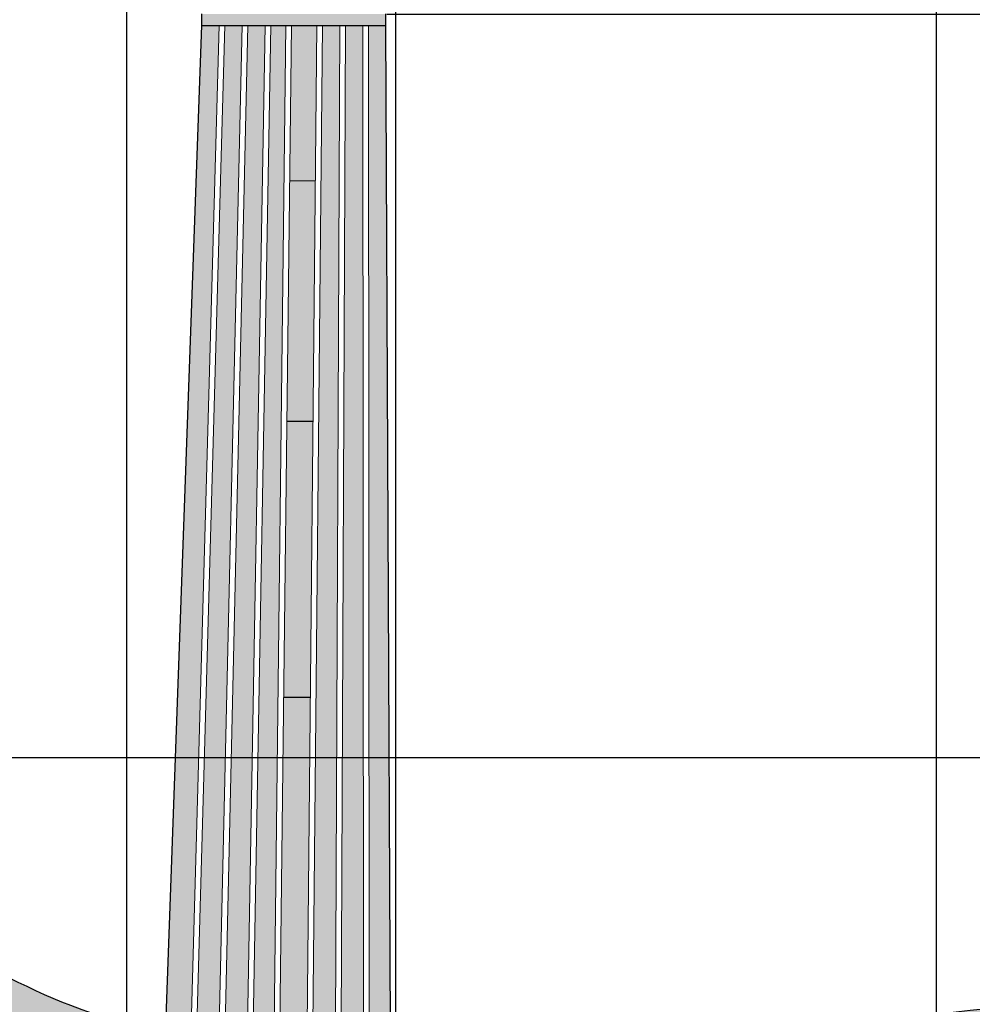
# Model space of a CAD drawing. Units: millimetres. Extents: x 11032 to 26788, y 3406 to 24505.
# Tile 76 of 78: x 16895 to 21051, y 17443 to 21738. Entities that reach past the tile are written whole.
import ezdxf

# ---------------------------------------------------------------- set-up
doc = ezdxf.new("R2010")
doc.units = ezdxf.units.MM
doc.header["$MEASUREMENT"] = 0
for name, color, linetype, lineweight in [('A-ANNO-DIMS', 2, 'Continuous', 18), ('A-ELEV-NECK', 7, 'Continuous', 25), ('A-ELEV-STRG', 7, 'Continuous', 13), ('A-ROOF', 7, 'Continuous', 30)]:
    doc.layers.add(name, color=color, linetype=linetype, lineweight=lineweight)
for name, color, linetype, lineweight, true_color in [('A-ELEV-NECK-PATT', 159, 'Continuous', 13, 0x22346e), ('A-ELEV-TUNE-PATT', 251, 'Continuous', 13, 0x636466), ('A-ROOF-PATT', 9, 'Continuous', 13, 0xc7c8ca)]:
    doc.layers.add(name, color=color, linetype=linetype, lineweight=lineweight, true_color=true_color)
doc.styles.get("Standard").update_dxf_attribs({"font": 'arial.ttf'})
doc.dimstyles.get("Standard").update_dxf_attribs({"dimtxt": 150, "dimasz": 100, "dimexe": 10, "dimexo": 5, "dimgap": 5, "dimtad": 0, "dimtih": 1, "dimtoh": 1, "dimdec": 0, "dimzin": 0, "dimdsep": 46, "dimtxsty": 'Standard', "dimcen": 0.09, "dimadec": 0, "dimazin": 0, "dimtfac": 1, "dimtdec": 0, "dimtofl": 0, "dimtmove": 0, "dimatfit": 3, "dimfxl": 1, "dimtolj": 1, "dimtzin": 0, "dimarcsym": 0})

# ---------------------------------------------------------------- blocks, each defined once
blk = doc.blocks.new('*D28')
at = {"layer": 'A-ANNO-DIMS', "color": 0, "lineweight": -2, "transparency": 16777216}
for p, q in [((17252.8, 22072.2), (17252.8, 22172.2)), ((17252.8, 22172.2), (17352.8, 22172.2)), ((17289.8, 22072.2), (17242.8, 22072.2)), ((17252.8, 21892.4), (17252.8, 21972.2)), ((17289.8, 21792.4), (17242.8, 21792.4))]:
    blk.add_line(p, q, dxfattribs=at)
at = {"layer": 'A-ANNO-DIMS', "color": 0, "transparency": 16777216}
for points in [[(17236.2, 21972.2), (17269.5, 21972.2), (17252.8, 22072.2)], [(17236.2, 21892.4), (17269.5, 21892.4), (17252.8, 21792.4)]]:
    blk.add_solid(points, dxfattribs=at)
at = {"layer": 'Defpoints', "color": 0, "transparency": 16777216}
for p in [(17252.8, 22072.2), (17294.8, 22072.2), (17294.8, 21792.4)]:
    blk.add_point(p, dxfattribs=at)
at = {"layer": 'A-ANNO-DIMS', "color": 0, "transparency": 16777216, "insert": (18452.5, 22172.2), "char_height": 150, "attachment_point": 5}
blk.add_mtext('\\A1;TUNING KEY 280 TYP.', dxfattribs=at)
blk = doc.blocks.new('*D36')
at = {"layer": 'A-ANNO-DIMS', "color": 0, "lineweight": -2, "transparency": 16777216}
for p, q in [((12301.3, 17115.9), (12301.3, 24416.9)), ((12401.3, 24406.9), (18569.2, 24406.9)), ((25297.4, 24406.9), (19129.5, 24406.9)), ((25397.4, 4466.4), (25397.4, 24416.9))]:
    blk.add_line(p, q, dxfattribs=at)
at = {"layer": 'A-ANNO-DIMS', "color": 0, "transparency": 16777216}
for points in [[(12401.3, 24423.5), (12401.3, 24390.2), (12301.3, 24406.9)], [(25297.4, 24423.5), (25297.4, 24390.2), (25397.4, 24406.9)]]:
    blk.add_solid(points, dxfattribs=at)
at = {"layer": 'Defpoints', "color": 0, "transparency": 16777216}
for p in [(25397.4, 24406.9), (12301.3, 17110.9), (25397.4, 4461.4)]:
    blk.add_point(p, dxfattribs=at)
at = {"layer": 'A-ANNO-DIMS', "color": 0, "transparency": 16777216, "insert": (18849.3, 24406.9), "char_height": 150, "attachment_point": 5}
blk.add_mtext('\\A1;13096', dxfattribs=at)
blk = doc.blocks.new('*D37')
at = {"layer": 'A-ANNO-DIMS', "color": 0, "lineweight": -2, "transparency": 16777216}
for p, q in [((18087.7, 23450.4), (11334.8, 23450.4)), ((11344.8, 23350.4), (11344.8, 14037.5)), ((11344.8, 4561.4), (11344.8, 13874.3)), ((12927.7, 4461.4), (11334.8, 4461.4))]:
    blk.add_line(p, q, dxfattribs=at)
at = {"layer": 'A-ANNO-DIMS', "color": 0, "transparency": 16777216}
for points in [[(11328.1, 23350.4), (11361.4, 23350.4), (11344.8, 23450.4)], [(11328.1, 4561.4), (11361.4, 4561.4), (11344.8, 4461.4)]]:
    blk.add_solid(points, dxfattribs=at)
at = {"layer": 'Defpoints', "color": 0, "transparency": 16777216}
for p in [(11344.8, 23450.4), (18092.7, 23450.4), (12932.7, 4461.4)]:
    blk.add_point(p, dxfattribs=at)
at = {"layer": 'A-ANNO-DIMS', "color": 0, "transparency": 16777216, "insert": (11344.8, 13955.9), "char_height": 150, "attachment_point": 5}
blk.add_mtext('\\A1;18989', dxfattribs=at)
blk = doc.blocks.new('*D45')
at = {"layer": 'A-ANNO-DIMS', "color": 0, "lineweight": -2, "transparency": 16777216}
for p, q in [((13792.4, 18518.9), (26363.9, 18518.9)), ((26353.9, 18418.9), (26353.9, 17450.3)), ((26353.9, 16318.4), (26353.9, 17287)), ((22902.4, 16218.4), (26363.9, 16218.4))]:
    blk.add_line(p, q, dxfattribs=at)
at = {"layer": 'A-ANNO-DIMS', "color": 0, "transparency": 16777216}
for points in [[(26337.2, 18418.9), (26370.6, 18418.9), (26353.9, 18518.9)], [(26337.2, 16318.4), (26370.6, 16318.4), (26353.9, 16218.4)]]:
    blk.add_solid(points, dxfattribs=at)
at = {"layer": 'Defpoints', "color": 0, "transparency": 16777216}
for p in [(13787.4, 18518.9), (26353.9, 18518.9), (22897.4, 16218.4)]:
    blk.add_point(p, dxfattribs=at)
at = {"layer": 'A-ANNO-DIMS', "color": 0, "transparency": 16777216, "insert": (26353.9, 17368.7), "char_height": 150, "attachment_point": 5}
blk.add_mtext('\\A1;2300.5', dxfattribs=at)
blk = doc.blocks.new('*D46')
at = {"layer": 'A-ANNO-DIMS', "color": 0, "lineweight": -2, "transparency": 16777216}
for p, q in [((18497.2, 21762.9), (26363.9, 21762.9)), ((26353.9, 21662.9), (26353.9, 20222.6)), ((26353.9, 18618.9), (26353.9, 20059.3)), ((13792.4, 18518.9), (26363.9, 18518.9))]:
    blk.add_line(p, q, dxfattribs=at)
at = {"layer": 'A-ANNO-DIMS', "color": 0, "transparency": 16777216}
for points in [[(26337.2, 21662.9), (26370.6, 21662.9), (26353.9, 21762.9)], [(26337.2, 18618.9), (26370.6, 18618.9), (26353.9, 18518.9)]]:
    blk.add_solid(points, dxfattribs=at)
at = {"layer": 'Defpoints', "color": 0, "transparency": 16777216}
for p in [(18492.2, 21762.9), (26353.9, 21762.9), (13787.4, 18518.9)]:
    blk.add_point(p, dxfattribs=at)
at = {"layer": 'A-ANNO-DIMS', "color": 0, "transparency": 16777216, "insert": (26353.9, 20140.9), "char_height": 150, "attachment_point": 5}
blk.add_mtext('\\A1;3244', dxfattribs=at)
blk = doc.blocks.new('*D57')
at = {"layer": 'A-ANNO-DIMS', "color": 0, "lineweight": -2, "transparency": 16777216}
for p, q in [((14994.7, 7266.4), (14994.7, 24416.9)), ((15094.7, 24406.9), (17716, 24406.9)), ((20794.7, 24406.9), (18173.4, 24406.9)), ((20894.7, 7266.4), (20894.7, 24416.9))]:
    blk.add_line(p, q, dxfattribs=at)
at = {"layer": 'A-ANNO-DIMS', "color": 0, "transparency": 16777216}
for points in [[(15094.7, 24423.5), (15094.7, 24390.2), (14994.7, 24406.9)], [(20794.7, 24423.5), (20794.7, 24390.2), (20894.7, 24406.9)]]:
    blk.add_solid(points, dxfattribs=at)
at = {"layer": 'Defpoints', "color": 0, "transparency": 16777216}
for p in [(20894.7, 24406.9), (14994.7, 7261.4), (20894.7, 7261.4)]:
    blk.add_point(p, dxfattribs=at)
at = {"layer": 'A-ANNO-DIMS', "color": 0, "transparency": 16777216, "insert": (17944.7, 24406.9), "char_height": 150, "attachment_point": 5}
blk.add_mtext('\\A1;5900', dxfattribs=at)
blk = doc.blocks.new('*D65')
at = {"layer": 'A-ANNO-DIMS', "color": 0, "lineweight": -2, "transparency": 16777216}
for p, q in [((17362, 12566.3), (17362, 24416.9)), ((17462, 24406.9), (17639.4, 24406.9)), ((18435.4, 24406.9), (18258, 24406.9)), ((18535.4, 12566.5), (18535.4, 24416.9))]:
    blk.add_line(p, q, dxfattribs=at)
at = {"layer": 'A-ANNO-DIMS', "color": 0, "transparency": 16777216}
for points in [[(17462, 24423.5), (17462, 24390.2), (17362, 24406.9)], [(18435.4, 24423.5), (18435.4, 24390.2), (18535.4, 24406.9)]]:
    blk.add_solid(points, dxfattribs=at)
at = {"layer": 'Defpoints', "color": 0, "transparency": 16777216}
for p in [(18535.4, 24406.9), (17362, 12561.3), (18535.4, 12561.5)]:
    blk.add_point(p, dxfattribs=at)
at = {"layer": 'A-ANNO-DIMS', "color": 0, "transparency": 16777216, "insert": (17948.7, 24406.9), "char_height": 150, "attachment_point": 5}
blk.add_mtext('\\A1;1173.3', dxfattribs=at)

msp = doc.modelspace()

# ---------------------------------------------------------------- hatches: boundary and pattern name
at = {"layer": 'A-ELEV-NECK-PATT'}
h = msp.add_hatch(color=256, dxfattribs=at)
h.set_gradient(color1=(82, 15, 16), color2=(153, 76, 0), name='INVHEMISPHERICAL')
edge = h.paths.add_edge_path()
edge.add_line((17765.577, 21712.945), (17690.161, 21712.945))
edge.add_line((17690.161, 21712.945), (17532.827, 17324.837))
edge.add_spline(control_points=[(17532.827, 17324.837), (17568.929, 17318.668), (17605.243, 17313.31), (17641.798, 17308.706)], knot_values=[8560.66857913, 8560.66857913, 8560.66857913, 8560.66857913, 8678.18536837, 8678.18536837, 8678.18536837, 8678.18536837], degree=3, periodic=0)
edge.add_line((17641.798, 17308.706), (17765.577, 21712.945))
edge = h.paths.add_edge_path()
edge.add_spline(control_points=[(17666.718, 17305.687), (17699.249, 17301.903), (17731.975, 17298.702), (17764.917, 17296.043)], knot_values=[8704.84912349, 8704.84912349, 8704.84912349, 8704.84912349, 8809.1081873, 8809.1081873, 8809.1081873, 8809.1081873], degree=3, periodic=0)
edge.add_line((17764.917, 17296.043), (17865.857, 21712.945))
edge.add_line((17865.857, 21712.945), (17790.586, 21712.945))
edge.add_line((17790.586, 21712.945), (17666.718, 17305.687))
edge = h.paths.add_edge_path()
edge.add_line((17966.114, 21712.945), (17890.863, 21712.945))
edge.add_line((17890.863, 21712.945), (17789.878, 17294.135))
edge.add_spline(control_points=[(17789.878, 17294.135), (17822.446, 17291.782), (17855.23, 17289.947), (17888.249, 17288.59)], knot_values=[8835.39626479, 8835.39626479, 8835.39626479, 8835.39626479, 8938.12522047, 8938.12522047, 8938.12522047, 8938.12522047], degree=3, periodic=0)
edge.add_line((17888.249, 17288.59), (17966.114, 21712.945))
h = msp.add_hatch(color=256, dxfattribs=at)
h.set_gradient(color1=(82, 15, 16), color2=(153, 76, 0), name='INVHEMISPHERICAL')
edge = h.paths.add_edge_path()
edge.add_line((18055.913, 21712.945), (17991.118, 21712.945))
edge.add_line((17991.118, 21712.945), (17913.235, 17287.655))
edge.add_spline(control_points=[(17913.235, 17287.655), (17923.7, 17287.302), (17934.19, 17286.996), (17944.704, 17286.735)], knot_values=[8963.99017486, 8963.99017486, 8963.99017486, 8963.99017486, 8996.4318779, 8996.4318779, 8996.4318779, 8996.4318779], degree=3, periodic=0)
edge.add_spline(control_points=[(17944.704, 17286.735), (17964.82, 17285.722), (17984.935, 17284.709), (18005.051, 17283.703)], knot_values=[0, 0, 0, 0, 60.41749209, 60.41749209, 60.41749209, 60.41749209], degree=3, periodic=0)
edge.add_line((18005.051, 17283.703), (18055.913, 21712.945))
edge = h.paths.add_edge_path()
edge.add_line((18492.19, 21712.945), (18416.998, 21712.945))
edge.add_line((18416.998, 21712.945), (18420.504, 17266.134))
edge.add_spline(control_points=[(18420.504, 17266.134), (18451.394, 17265.216), (18482.287, 17264.397), (18513.182, 17263.662)], knot_values=[476.26006783, 476.26006783, 476.26006783, 476.26006783, 568.98430855, 568.98430855, 568.98430855, 568.98430855], degree=3, periodic=0)
edge.add_line((18513.182, 17263.662), (18492.19, 21712.945))
edge = h.paths.add_edge_path()
edge.add_spline(control_points=[(18296.914, 17270.367), (18316.656, 17269.603), (18349.518, 17268.396), (18382.383, 17267.313), (18395.503, 17266.9)], knot_values=[352.58081587, 352.58081587, 352.58081587, 352.58081587, 411.85892504, 451.24395945, 451.24395945, 451.24395945, 451.24395945], degree=3, periodic=0)
edge.add_line((18395.503, 17266.9), (18391.999, 21712.945))
edge.add_line((18391.999, 21712.945), (18316.752, 21712.945))
edge.add_line((18316.752, 21712.945), (18296.914, 17270.367))
edge = h.paths.add_edge_path()
edge.add_line((18291.755, 21712.945), (18216.518, 21712.945))
edge.add_line((18216.518, 21712.945), (18173.381, 17275.594))
edge.add_spline(control_points=[(18173.381, 17275.594), (18206.225, 17274.101), (18239.071, 17272.678), (18271.92, 17271.355)], knot_values=[228.93242669, 228.93242669, 228.93242669, 228.93242669, 327.56540209, 327.56540209, 327.56540209, 327.56540209], degree=3, periodic=0)
edge.add_line((18271.92, 17271.355), (18291.755, 21712.945))
h = msp.add_hatch(color=256, dxfattribs=at)
h.set_gradient(color1=(82, 15, 16), color2=(153, 76, 0), name='INVCURVED')
h.paths.add_polyline_path([(18047.271, 18783.21), (18163.029, 18782.085), (18174.733, 19985.929), (18061.095, 19987.033)])
h.paths.add_polyline_path([(18184.929, 21034.754), (18073.138, 21035.841), (18061.095, 19987.033), (18174.733, 19985.929)])
h.paths.add_polyline_path([(18073.138, 21035.841), (18184.929, 21034.754), (18191.522, 21712.945), (18080.914, 21712.945)])
h = msp.add_hatch(color=256, dxfattribs=at)
h.set_gradient(color1=(82, 15, 16), color2=(153, 76, 0), name='INVCURVED')
edge = h.paths.add_edge_path()
edge.add_spline(control_points=[(18030.038, 17282.457), (18069.489, 17280.497), (18108.941, 17278.575), (18148.395, 17276.742)], knot_values=[85.43243603, 85.43243603, 85.43243603, 85.43243603, 203.92020001, 203.92020001, 203.92020001, 203.92020001], degree=3, periodic=0)
edge.add_line((18148.395, 17276.742), (18163.029, 18782.085))
edge.add_line((18163.029, 18782.085), (18047.271, 18783.21))
edge.add_line((18047.271, 18783.21), (18030.038, 17282.457))
at = {"layer": 'A-ELEV-TUNE-PATT'}
msp.add_hatch(color=256, dxfattribs=at).paths.add_polyline_path([(18492.19, 21762.945), (17690.161, 21762.945), (17690.161, 21712.945), (18055.913, 21712.945), (18055.916, 21713.232), (18492.19, 21712.945)])
at = {"layer": 'A-ROOF-PATT'}
h = msp.add_hatch(color=256, dxfattribs=at)
edge = h.paths.add_edge_path()
edge.add_spline(control_points=[(17532.827, 17324.837), (17391.335, 17349.016), (16840.872, 17494.912), (16080.055, 18069.544), (14738.803, 18299.641), (13382.429, 18838.336), (12580.532, 17870.207), (12430.422, 17563.822)], knot_values=[2977.60279446, 2977.60279446, 2977.60279446, 2977.60279446, 3438.18406011, 4811.64630219, 5622.86754827, 7588.02881883, 8560.66857913, 8560.66857913, 8560.66857913, 8560.66857913], degree=3, periodic=0)
edge.add_spline(control_points=[(12430.422, 17563.822), (12437.904, 17573.36), (12445.386, 17582.899), (12452.869, 17592.437), (12452.869, 17592.438), (12452.869, 17592.438), (12452.869, 17592.438)], knot_values=[1408.56413798, 1408.56413798, 1408.56413798, 1408.56413798, 1444.85989, 1444.85989, 1444.85989, 1444.86011829, 1444.86011829, 1444.86011829, 1444.86011829], degree=3, periodic=0)
edge.add_spline(control_points=[(12452.869, 17592.438), (12555.432, 17723.185), (12736.557, 17929.686), (13044.86, 18114.643), (13219.943, 18189.644), (13299.92, 18220.646)], knot_values=[339.31824597, 339.31824597, 339.31824597, 339.31824597, 836.83499673, 1151.25129334, 1408.56413798, 1408.56413798, 1408.56413798, 1408.56413798], degree=3, periodic=0)
edge.add_spline(control_points=[(13299.92, 18220.646), (13299.998, 18220.689), (13300.077, 18220.732), (13319.738, 18231.488), (13339.24, 18241.402), (13388.645, 18264.703), (13418.466, 18277.069), (13478.019, 18298.648), (13507.751, 18307.861), (13544.561, 18317.488), (13551.584, 18319.245), (13558.612, 18320.924)], knot_values=[3783.89509717, 3783.89509717, 3783.89509717, 3783.89509717, 3784.1737101, 3784.1737101, 3853.4666747, 3853.4666747, 3960.24019172, 3960.24019172, 4067.01370874, 4067.01370874, 4092.17446487, 4092.17446487, 4092.17446487, 4092.17446487], degree=3, periodic=0)
edge.add_spline(control_points=[(13558.612, 18320.924), (13581.407, 18326.373), (13604.25, 18331.007), (13657.184, 18339.957), (13687.338, 18343.732), (13748.098, 18348.892), (13778.704, 18350.276), (13840.46, 18350.833), (13871.609, 18350.005), (13934.496, 18346.313), (13966.232, 18343.449), (14030.297, 18335.871), (14062.625, 18331.158), (14127.853, 18320.088), (14160.753, 18313.73), (14241.357, 18296.556), (14289.343, 18284.997), (14386.31, 18259.688), (14435.291, 18245.941), (14534.161, 18217.034), (14584.049, 18201.875), (14684.682, 18170.964), (14735.427, 18155.212), (14837.763, 18123.971), (14889.354, 18108.482), (14954.971, 18089.677), (14968.586, 18085.823), (14992.391, 18079.184), (15002.566, 18076.376), (15021.739, 18071.153), (15030.731, 18068.729), (15047.707, 18064.21), (15055.694, 18062.106), (15079.815, 18055.825), (15095.905, 18051.728), (15143.966, 18039.717), (15175.729, 18032.084), (15254.84, 18013.501), (15301.798, 18002.866), (15394.186, 17981.845), (15439.615, 17971.459), (15528.833, 17950.135), (15572.62, 17939.197), (15658.477, 17916.021), (15700.546, 17903.785), (15753.633, 17886.734), (15765.446, 17882.835), (15786.574, 17875.653), (15795.915, 17872.404), (15810.108, 17867.349), (15814.99, 17865.588), (15824.736, 17862.029), (15829.611, 17860.226), (15844.241, 17854.75), (15854.002, 17851.008), (15883.312, 17839.521), (15902.885, 17831.512), (15966.355, 17804.548), (16010.39, 17784.302), (16098.838, 17741.267), (16143.25, 17718.478), (16232.497, 17671.098), (16277.332, 17646.507), (16367.515, 17596.295), (16412.862, 17570.676), (16504.202, 17519.209), (16550.194, 17493.362), (16643.009, 17442.263), (16689.831, 17417.011), (16756.517, 17382.472), (16775.937, 17372.58), (16795.455, 17362.84)], knot_values=[4092.17446487, 4092.17446487, 4092.17446487, 4092.17446487, 4173.78722577, 4173.78722577, 4280.56074279, 4280.56074279, 4387.33425981, 4387.33425981, 4494.10777683, 4494.10777683, 4600.88129386, 4600.88129386, 4707.65481088, 4707.65481088, 4814.4283279, 4814.4283279, 4967.12624049, 4967.12624049, 5119.82415308, 5119.82415308, 5272.52206566, 5272.52206566, 5425.21997825, 5425.21997825, 5577.91789084, 5577.91789084, 5617.78533194, 5617.78533194, 5647.46484794, 5647.46484794, 5673.61102495, 5673.61102495, 5696.74760695, 5696.74760695, 5743.68189033, 5743.68189033, 5837.55045709, 5837.55045709, 5979.72610459, 5979.72610459, 6121.90175208, 6121.90175208, 6264.07739957, 6264.07739957, 6406.25304706, 6406.25304706, 6447.25858494, 6447.25858494, 6480.04208821, 6480.04208821, 6497.30770621, 6497.30770621, 6514.5733242, 6514.5733242, 6549.10456019, 6549.10456019, 6618.16703217, 6618.16703217, 6772.66101707, 6772.66101707, 6927.15500198, 6927.15500198, 7081.64898689, 7081.64898689, 7236.1429718, 7236.1429718, 7390.6369567, 7390.6369567, 7545.13094161, 7545.13094161, 7608.19928683, 7608.19928683, 7608.19928683, 7608.19928683], degree=3, periodic=0)
edge.add_spline(control_points=[(16795.455, 17362.84), (16814.335, 17349.456), (16832.897, 17336.263), (16873.225, 17307.197), (16894.778, 17291.386), (16936.221, 17259.941), (16956.11, 17244.308), (16993.863, 17213.094), (17011.726, 17197.514), (17041.993, 17169.265), (17054.791, 17156.601), (17078.762, 17131.225), (17089.933, 17118.516), (17110.618, 17092.991), (17120.131, 17080.178), (17130.17, 17065.264), (17131.487, 17063.277), (17133.77, 17059.776), (17134.746, 17058.261), (17136.69, 17055.205), (17137.657, 17053.668), (17140.539, 17049.025), (17142.438, 17045.89), (17148.068, 17036.367), (17151.732, 17029.859), (17163.03, 17008.788), (17170.335, 16993.646), (17184.087, 16961.978), (17190.534, 16945.453), (17202.562, 16911.165), (17208.142, 16893.402), (17218.448, 16856.821), (17223.173, 16838.003), (17231.801, 16799.51), (17235.705, 16779.837), (17241.533, 16746.739), (17243.676, 16733.5), (17247.718, 16706.37), (17249.608, 16692.472), (17252.066, 16672.69), (17252.761, 16666.875), (17254.1, 16655.226), (17254.744, 16649.4), (17256.596, 16631.917), (17257.727, 16620.254), (17260.823, 16585.238), (17262.489, 16561.858), (17266.551, 16488.654), (17267.658, 16438.661), (17267.349, 16375.228), (17267.193, 16362.07), (17266.95, 16348.891)], knot_values=[15.11304723, 15.11304723, 15.11304723, 15.11304723, 82.69951457, 82.69951457, 165.39902914, 165.39902914, 248.09854371, 248.09854371, 330.79805828, 330.79805828, 397.94194582, 397.94194582, 465.08583335, 465.08583335, 532.22972088, 532.22972088, 542.53374101, 542.53374101, 550.35681582, 550.35681582, 558.17989062, 558.17989062, 573.82604024, 573.82604024, 605.11833946, 605.11833946, 672.76406143, 672.76406143, 740.4097834, 740.4097834, 808.05550537, 808.05550537, 875.70122735, 875.70122735, 943.34694932, 943.34694932, 987.66134917, 987.66134917, 1033.41216123, 1033.41216123, 1052.38508762, 1052.38508762, 1071.35801402, 1071.35801402, 1109.30386682, 1109.30386682, 1185.19557241, 1185.19557241, 1346.44190265, 1346.44190265, 1388.55866312, 1388.55866312, 1388.55866312, 1388.55866312], degree=3, periodic=0)
edge.add_spline(control_points=[(17266.95, 16348.891), (17266.95, 16348.891), (17266.95, 16348.891), (17266.95, 16348.891), (17253.182, 15602.417), (17239.414, 14855.943), (17225.646, 14109.469)], knot_values=[1388.55866312, 1388.55866312, 1388.55866312, 1388.55866312, 1388.55896543, 1388.55896543, 1388.55896543, 3774.07676609, 3774.07676609, 3774.07676609, 3774.07676609], degree=3, periodic=0)
edge.add_spline(control_points=[(17225.646, 14109.469), (17226.198, 14109.827), (17226.748, 14110.185), (17242.065, 14120.191), (17255.956, 14130.116), (17274.422, 14144.286), (17279.609, 14148.386), (17284.686, 14152.511)], knot_values=[1926.3423968, 1926.3423968, 1926.3423968, 1926.3423968, 1927.31672898, 1927.31672898, 1953.51217613, 1953.51217613, 1964.07323478, 1964.07323478, 1964.07323478, 1964.07323478], degree=3, periodic=0)
edge.add_spline(control_points=[(17284.686, 14152.511), (17315.791, 14194.761), (17384.413, 14446.273), (17407.128, 14793.401), (17407.093, 15295.84), (17423.274, 15626.362), (17415.601, 15782.507)], knot_values=[0, 0, 0, 0, 163.25546741, 619.22967667, 1171.8624483, 1621.63555623, 1621.63555623, 1621.63555623, 1621.63555623], degree=3, periodic=0)
edge.add_spline(control_points=[(17415.601, 15782.507), (17438.21, 16077.57), (17410.495, 16533.484), (17390.893, 17030.649), (17301.082, 17169.349)], knot_values=[543.97847526, 543.97847526, 543.97847526, 543.97847526, 1452.98527668, 1960.01149261, 1960.01149261, 1960.01149261, 1960.01149261], degree=3, periodic=0)
edge.add_spline(control_points=[(17301.082, 17169.349), (17346.58, 17157.64), (17392.235, 17147.336), (17467.161, 17132.609), (17496.336, 17127.412), (17525.58, 17122.709)], knot_values=[8131.59393903, 8131.59393903, 8131.59393903, 8131.59393903, 8269.73492727, 8269.73492727, 8357.5016646, 8357.5016646, 8357.5016646, 8357.5016646], degree=3, periodic=0)
edge.add_line((17525.58, 17122.709), (17532.827, 17324.837))
edge = h.paths.add_edge_path(flags=17)
edge.add_spline(control_points=[(13340.537, 14602.706), (13316.172, 14726.456), (13323.666, 14932.342), (13637.836, 15081.117), (13863.248, 15171.051), (14002.1, 15224.503), (14058.539, 15244.876)], knot_values=[680.89318617, 680.89318617, 680.89318617, 680.89318617, 1033.47282894, 1337.40083264, 1604.72142636, 1784.29447217, 1784.29447217, 1784.29447217, 1784.29447217], degree=3, periodic=0)
edge.add_spline(control_points=[(14058.539, 15244.876), (14058.289, 15275.236), (14057.634, 15305.434), (14055.312, 15376.527), (14053.359, 15417.248), (14048.642, 15497.048), (14045.89, 15536.143), (14042.888, 15574.619)], knot_values=[6573.10654186, 6573.10654186, 6573.10654186, 6573.10654186, 6636.73300118, 6636.73300118, 6723.88905466, 6723.88905466, 6809.63287714, 6809.63287714, 6809.63287714, 6809.63287714], degree=3, periodic=0)
edge.add_spline(control_points=[(14042.888, 15574.619), (13546.54, 15403.221), (13074.735, 15143.241), (13277.36, 14695.339), (13340.537, 14602.706)], knot_values=[503.79257829, 503.79257829, 503.79257829, 503.79257829, 1728.17876056, 2051.34843998, 2051.34843998, 2051.34843998, 2051.34843998], degree=3, periodic=0)
h = msp.add_hatch(color=256, dxfattribs=at)
h.set_gradient(color1=(254, 234, 185), color2=(254, 204, 102), name='HEMISPHERICAL')
edge = h.paths.add_edge_path()
edge.add_line((15084.393, 17001.32), (15284.393, 17051.32))
edge.add_line((15284.393, 17051.32), (15470.537, 16752.334))
edge.add_spline(control_points=[(15470.537, 16752.334), (15683.311, 16831.508), (16106.827, 16912.335), (16625.609, 16876.997), (17083.498, 16357.78), (17257.801, 16180.113)], knot_values=[0, 0, 0, 0, 655.29363337, 1252.01578382, 1989.61628586, 1989.61628586, 1989.61628586, 1989.61628586], degree=3, periodic=0)
edge.add_spline(control_points=[(17257.801, 16180.113), (17260.851, 16236.372), (17263.9, 16292.632), (17266.95, 16348.891)], knot_values=[1132.9967717, 1132.9967717, 1132.9967717, 1132.9967717, 1198.04642249, 1198.04642249, 1198.04642249, 1198.04642249], degree=3, periodic=0)
edge.add_spline(control_points=[(17266.95, 16348.891), (17267.193, 16362.07), (17267.349, 16375.228), (17267.658, 16438.661), (17266.551, 16488.654), (17262.489, 16561.858), (17260.823, 16585.238), (17257.727, 16620.254), (17256.596, 16631.917), (17254.744, 16649.4), (17254.1, 16655.226), (17252.761, 16666.875), (17252.066, 16672.69), (17249.608, 16692.472), (17247.718, 16706.37), (17243.676, 16733.5), (17241.533, 16746.739), (17235.705, 16779.837), (17231.801, 16799.51), (17223.173, 16838.003), (17218.448, 16856.821), (17208.142, 16893.402), (17202.562, 16911.165), (17190.534, 16945.453), (17184.087, 16961.978), (17170.335, 16993.646), (17163.03, 17008.788), (17151.732, 17029.859), (17148.068, 17036.367), (17142.438, 17045.89), (17140.539, 17049.025), (17137.657, 17053.668), (17136.69, 17055.205), (17134.746, 17058.261), (17133.77, 17059.776), (17131.487, 17063.277), (17130.17, 17065.264), (17120.131, 17080.178), (17110.618, 17092.991), (17089.933, 17118.516), (17078.762, 17131.225), (17054.791, 17156.601), (17041.993, 17169.265), (17011.726, 17197.514), (16993.863, 17213.094), (16956.11, 17244.308), (16936.221, 17259.941), (16894.778, 17291.386), (16873.225, 17307.197), (16832.897, 17336.263), (16814.335, 17349.456), (16795.455, 17362.84)], knot_values=[15.11304723, 15.11304723, 15.11304723, 15.11304723, 57.2298077, 57.2298077, 218.47613793, 218.47613793, 294.36784353, 294.36784353, 332.31369632, 332.31369632, 351.28662272, 351.28662272, 370.25954912, 370.25954912, 416.01036118, 416.01036118, 460.32476103, 460.32476103, 527.970483, 527.970483, 595.61620497, 595.61620497, 663.26192694, 663.26192694, 730.90764891, 730.90764891, 798.55337089, 798.55337089, 829.84567011, 829.84567011, 845.49181972, 845.49181972, 853.31489453, 853.31489453, 861.13796933, 861.13796933, 871.44198947, 871.44198947, 938.585877, 938.585877, 1005.72976453, 1005.72976453, 1072.87365206, 1072.87365206, 1155.57316663, 1155.57316663, 1238.2726812, 1238.2726812, 1320.97219578, 1320.97219578, 1388.55866312, 1388.55866312, 1388.55866312, 1388.55866312], degree=3, periodic=0)
edge.add_spline(control_points=[(16795.455, 17362.84), (16775.937, 17372.58), (16756.517, 17382.472), (16689.831, 17417.011), (16643.009, 17442.263), (16550.194, 17493.362), (16504.202, 17519.209), (16412.862, 17570.676), (16367.515, 17596.295), (16277.332, 17646.507), (16232.497, 17671.098), (16143.25, 17718.478), (16098.838, 17741.267), (16010.39, 17784.302), (15966.355, 17804.548), (15902.885, 17831.512), (15883.312, 17839.521), (15854.002, 17851.008), (15844.241, 17854.75), (15829.611, 17860.226), (15824.736, 17862.029), (15814.99, 17865.588), (15810.108, 17867.349), (15795.915, 17872.404), (15786.574, 17875.653), (15765.446, 17882.835), (15753.633, 17886.734), (15700.546, 17903.785), (15658.477, 17916.021), (15572.62, 17939.197), (15528.833, 17950.135), (15439.615, 17971.459), (15394.186, 17981.845), (15301.798, 18002.866), (15254.84, 18013.501), (15175.729, 18032.084), (15143.966, 18039.717), (15095.905, 18051.728), (15079.815, 18055.825), (15055.694, 18062.106), (15047.707, 18064.21), (15030.731, 18068.729), (15021.739, 18071.153), (15002.566, 18076.376), (14992.391, 18079.184), (14968.586, 18085.823), (14954.971, 18089.677), (14889.354, 18108.482), (14837.763, 18123.971), (14735.427, 18155.212), (14684.682, 18170.964), (14584.049, 18201.875), (14534.161, 18217.034), (14435.291, 18245.941), (14386.31, 18259.688), (14289.343, 18284.997), (14241.357, 18296.556), (14160.753, 18313.73), (14127.853, 18320.088), (14062.625, 18331.158), (14030.297, 18335.871), (13966.232, 18343.449), (13934.496, 18346.313), (13871.609, 18350.005), (13840.46, 18350.833), (13778.704, 18350.276), (13748.098, 18348.892), (13687.338, 18343.732), (13657.184, 18339.957), (13604.25, 18331.007), (13581.407, 18326.373), (13558.612, 18320.924)], knot_values=[4092.17446487, 4092.17446487, 4092.17446487, 4092.17446487, 4155.24281009, 4155.24281009, 4309.736795, 4309.736795, 4464.2307799, 4464.2307799, 4618.72476481, 4618.72476481, 4773.21874972, 4773.21874972, 4927.71273463, 4927.71273463, 5082.20671953, 5082.20671953, 5151.26919151, 5151.26919151, 5185.8004275, 5185.8004275, 5203.0660455, 5203.0660455, 5220.33166349, 5220.33166349, 5253.11516676, 5253.11516676, 5294.12070464, 5294.12070464, 5436.29635213, 5436.29635213, 5578.47199962, 5578.47199962, 5720.64764711, 5720.64764711, 5862.82329461, 5862.82329461, 5956.69186137, 5956.69186137, 6003.62614475, 6003.62614475, 6026.76272675, 6026.76272675, 6052.90890376, 6052.90890376, 6082.58841976, 6082.58841976, 6122.45586086, 6122.45586086, 6275.15377345, 6275.15377345, 6427.85168604, 6427.85168604, 6580.54959862, 6580.54959862, 6733.24751121, 6733.24751121, 6885.9454238, 6885.9454238, 6992.71894082, 6992.71894082, 7099.49245784, 7099.49245784, 7206.26597487, 7206.26597487, 7313.03949189, 7313.03949189, 7419.81300891, 7419.81300891, 7526.58652593, 7526.58652593, 7608.19928683, 7608.19928683, 7608.19928683, 7608.19928683], degree=3, periodic=0)
edge.add_spline(control_points=[(13558.612, 18320.924), (13472.381, 18287.498), (13386.15, 18254.072), (13299.92, 18220.646), (13299.92, 18220.646), (13299.92, 18220.646), (13299.92, 18220.646)], knot_values=[61.88324569, 61.88324569, 61.88324569, 61.88324569, 339.3179746, 339.3179746, 339.3179746, 339.31824597, 339.31824597, 339.31824597, 339.31824597], degree=3, periodic=0)
edge.add_spline(control_points=[(13299.92, 18220.646), (13219.943, 18189.644), (13044.86, 18114.643), (12736.557, 17929.686), (12555.432, 17723.185), (12452.869, 17592.438)], knot_values=[339.31824597, 339.31824597, 339.31824597, 339.31824597, 596.63109061, 911.04738723, 1408.56413798, 1408.56413798, 1408.56413798, 1408.56413798], degree=3, periodic=0)
edge.add_spline(control_points=[(12452.869, 17592.438), (12452.869, 17592.438), (12452.869, 17592.438), (12452.869, 17592.437), (12445.386, 17582.899), (12437.904, 17573.36), (12430.422, 17563.822)], knot_values=[1408.56413798, 1408.56413798, 1408.56413798, 1408.56413798, 1408.56436627, 1408.56436627, 1408.56436627, 1444.86011829, 1444.86011829, 1444.86011829, 1444.86011829], degree=3, periodic=0)
edge.add_spline(control_points=[(12430.422, 17563.822), (12373.797, 17448.248), (12157.302, 16836.764), (12751.985, 16393.69), (13424.325, 15907.903), (14042.888, 15574.619)], knot_values=[0, 0, 0, 0, 366.89930338, 1975.59410824, 2977.60279446, 2977.60279446, 2977.60279446, 2977.60279446], degree=3, periodic=0)
edge.add_spline(control_points=[(14042.888, 15574.619), (14042.839, 15575.252), (14042.789, 15575.886), (14039.681, 15615.607), (14036.366, 15654.052), (14029.551, 15729.305), (14026.05, 15766.114), (14019.175, 15837.686), (14015.8, 15872.45), (13903.823, 16338.596)], knot_values=[6310.22615039, 6310.22615039, 6310.22615039, 6310.22615039, 6311.63838141, 6311.63838141, 6398.79443489, 6398.79443489, 6485.95048837, 6485.95048837, 6573.10654186, 6573.10654186, 6573.10654186, 6573.10654186], degree=3, periodic=0)
edge.add_spline(control_points=[(13903.823, 16338.596), (14237.315, 16236.889), (14456.623, 16167.555), (14614.196, 16115.84)], knot_values=[0, 0, 0, 0, 202.98534191, 202.98534191, 202.98534191, 202.98534191], degree=3, periodic=0)
edge.add_spline(control_points=[(14614.196, 16115.84), (14663.209, 16178.992), (14799.965, 16341.237), (14969.915, 16481.426), (15084.393, 16556.825)], knot_values=[2405.03450449, 2405.03450449, 2405.03450449, 2405.03450449, 2644.88269663, 3039.27072715, 3039.27072715, 3039.27072715, 3039.27072715], degree=3, periodic=0)
edge.add_line((15084.393, 16556.825), (15084.393, 17001.32))
h.paths.add_polyline_path([(14195.599, 17606.181, -1), (14395.599, 17606.181, -1)], flags=16)
h.paths.add_polyline_path([(13310.178, 17032.97, -1), (13510.178, 17032.97, -1)], flags=16)
h = msp.add_hatch(color=256, dxfattribs=at)
edge = h.paths.add_edge_path()
edge.add_spline(control_points=[(18514.126, 17063.566), (18809.773, 17038.521), (19288.07, 16988.339), (19761.843, 17020.464), (19965.955, 17031.58)], knot_values=[0, 0, 0, 0, 871.48115533, 1383.18424693, 1383.18424693, 1383.18424693, 1383.18424693], degree=3, periodic=0)
edge.add_spline(control_points=[(19965.955, 17031.58), (20122.484, 17046.068), (20408.011, 17091.181), (20910.567, 17150.246), (21440.234, 17310.172), (21915.866, 17351.508), (22364.272, 17406.622), (22705.353, 17409.356), (22912.577, 17410.967), (22981.194, 17409.426)], knot_values=[0, 0, 0, 0, 414.81784697, 1085.22788952, 1556.54039253, 2003.31216232, 2520.51919616, 2899.47011217, 3092.27759325, 3092.27759325, 3092.27759325, 3092.27759325], degree=3, periodic=0)
edge.add_spline(control_points=[(22981.194, 17409.426), (23026.355, 17412.719), (23070.675, 17406.134), (23179.968, 17412.17), (23244.326, 17403.734), (23304.873, 17403.391)], knot_values=[11756.28081343, 11756.28081343, 11756.28081343, 11756.28081343, 11879.15309498, 11879.15309498, 12065.87545546, 12065.87545546, 12065.87545546, 12065.87545546], degree=3, periodic=0)
edge.add_spline(control_points=[(23304.873, 17403.391), (23443.416, 17391.278), (23687.5, 17400.339), (23988.629, 17323.661), (24193.084, 17226.949), (24257.37, 17136.735), (24279.347, 17098.191)], knot_values=[0, 0, 0, 0, 412.75172359, 727.19040018, 931.86025321, 1064.01641738, 1064.01641738, 1064.01641738, 1064.01641738], degree=3, periodic=0)
edge.add_spline(control_points=[(24279.347, 17098.191), (24276.632, 17112.026), (24103.56, 17784.539), (21679.83, 17482.933), (20092.886, 17311.864), (19886.51, 17298.161)], knot_values=[9435.32329041, 9435.32329041, 9435.32329041, 9435.32329041, 9511.54858978, 13244.41643911, 13837.11981978, 13837.11981978, 13837.11981978, 13837.11981978], degree=3, periodic=0)
edge.add_spline(control_points=[(19886.51, 17298.161), (19770.33, 17290.447), (19654.15, 17282.732), (19537.97, 17275.018), (19460.41, 17269.868), (19382.851, 17264.718), (19305.291, 17259.568)], knot_values=[8878.9087223, 8878.9087223, 8878.9087223, 8878.9087223, 9212.57342317, 9212.57342317, 9212.57342317, 9435.32303857, 9435.32303857, 9435.32303857, 9435.32303857], degree=3, periodic=0)
edge.add_spline(control_points=[(19305.291, 17259.568), (19183.371, 17255.041), (18919.19, 17257.277), (18655.158, 17260.282), (18513.182, 17263.662)], knot_values=[568.98430855, 568.98430855, 568.98430855, 568.98430855, 934.97323186, 1361.07600794, 1361.07600794, 1361.07600794, 1361.07600794], degree=3, periodic=0)
edge.add_line((18513.182, 17263.662), (18514.126, 17063.566))

# ---------------------------------------------------------------- linework, layer by layer
at = {"layer": 'A-ELEV-NECK'}
for p, q in [((17690.161, 21712.945), (17690.161, 21762.945)), ((18492.19, 21712.945), (18492.19, 21762.945)), ((17357.817, 12443.722), (17690.161, 21712.945)), ((17690.161, 21712.945), (18492.19, 21712.945)), ((18055.916, 21713.232), (18492.19, 21712.945)), ((18535.612, 12509.736), (18492.19, 21712.945)), ((18073.138, 21035.841), (18184.929, 21034.754)), ((18061.095, 19987.033), (18174.733, 19985.929)), ((18047.271, 18783.21), (18163.029, 18782.085))]:
    msp.add_line(p, q, dxfattribs=at)
at = {"layer": 'A-ELEV-STRG'}
for p, q in [((17449.067, 10451.016), (17765.577, 21712.945)), ((17474.065, 10451.016), (17790.586, 21712.945)), ((17608.488, 10451.016), (17865.857, 21712.945)), ((17633.488, 10451.016), (17890.863, 21712.945)), ((17767.913, 10451.016), (17966.114, 21712.945)), ((17792.914, 10451.016), (17991.118, 21712.945)), ((17926.591, 10451.016), (18055.916, 21713.232)), ((17951.591, 10451.016), (18080.917, 21713.216)), ((18082.038, 10451.016), (18191.524, 21713.143)), ((18107.038, 10451.016), (18216.519, 21713.127)), ((18241.462, 10451.016), (18291.755, 21713.077)), ((18266.462, 10451.016), (18316.752, 21713.061)), ((18400.876, 10451.016), (18391.999, 21713.011)), ((18425.878, 10451.016), (18416.998, 21712.995))]:
    msp.add_line(p, q, dxfattribs=at)
at = {"layer": 'A-ROOF'}
for points, knots in [([(14042.888, 15574.619), (13424.325, 15907.903), (12751.985, 16393.69), (11963.048, 16981.495), (13249.687, 18891.056), (14738.803, 18299.641), (16080.055, 18069.544), (16966.203, 17400.251), (17654.208, 17293.942), (17944.704, 17286.735)], [0, 0, 0, 0, 1002.00868622, 2610.70349108, 3950.24255476, 5915.40382532, 6726.62507141, 8100.08731348, 8996.4318779, 8996.4318779, 8996.4318779, 8996.4318779]), ([(19305.291, 17259.568), (19382.851, 17264.718), (19460.41, 17269.868), (19537.97, 17275.018), (19654.15, 17282.732), (19770.33, 17290.447), (19886.51, 17298.161), (19886.51, 17298.161), (19886.51, 17298.161), (19886.51, 17298.161), (20092.886, 17311.864), (21679.83, 17482.933), (25498.5, 17958.124), (23655.645, 15804.534), (22897.404, 14361.22)], [8878.9087223, 8878.9087223, 8878.9087223, 8878.9087223, 9101.65833771, 9101.65833771, 9101.65833771, 9435.32303857, 9435.32303857, 9435.32303857, 9435.32329041, 9435.32329041, 9435.32329041, 10028.02667108, 13760.8945204, 16370.50452639, 16370.50452639, 16370.50452639, 16370.50452639])]:
    msp.add_open_spline(points, degree=3, knots=knots, dxfattribs=at)

# ---------------------------------------------------------------- dimensions: what is measured, and where the dimension line sits
at = {"layer": 'A-ANNO-DIMS'}
for base, p1, p2, override, picture, middle in [((25397.404, 24406.858), (12301.265, 17110.885), (25397.404, 4461.399), {"dimdec": 0, "dimlfac": 1, "dimrnd": 0, "dimzin": 0, "dimdsep": 46, "dimlunit": 2}, '*D36', (18849.334, 24406.858)), ((20894.704, 24406.858), (14994.704, 7261.399), (20894.704, 7261.399), {"dimdec": 0, "dimlfac": 1, "dimrnd": 0, "dimzin": 0, "dimdsep": 46, "dimlunit": 2}, '*D57', (17944.704, 24406.858)), ((18535.366, 24406.858), (17362.033, 12561.3), (18535.366, 12561.507), {"dimdec": 1, "dimlfac": 1, "dimrnd": 0, "dimzin": 0, "dimdsep": 46, "dimlunit": 2}, '*D65', (17948.7, 24406.858))]:
    dim = msp.add_linear_dim(base=base, p1=p1, p2=p2, dimstyle='Standard', override=override, dxfattribs=at)
    dim.commit()
    dim.dimension.update_dxf_attribs({"geometry": picture, "text_midpoint": middle})
for base, p1, p2, override, picture, middle in [((11344.765, 23450.358), (12932.665, 4461.399), (18092.739, 23450.358), {"dimdec": 0, "dimlfac": 1, "dimrnd": 0, "dimzin": 0, "dimdsep": 46, "dimlunit": 2}, '*D37', (11344.765, 13955.879)), ((26353.904, 21762.945), (13787.367, 18518.925), (18492.19, 21762.945), {"dimdec": 0, "dimlfac": 1, "dimrnd": 0, "dimzin": 0, "dimdsep": 46, "dimlunit": 2}, '*D46', (26353.904, 20140.935)), ((26353.904, 18518.925), (22897.404, 16218.44), (13787.367, 18518.925), {"dimdec": 1, "dimlfac": 1, "dimrnd": 0, "dimzin": 0, "dimdsep": 46, "dimlunit": 2}, '*D45', (26353.904, 17368.682))]:
    dim = msp.add_linear_dim(base=base, p1=p1, p2=p2, angle=90, dimstyle='Standard', override=override, dxfattribs=at)
    dim.commit()
    dim.dimension.update_dxf_attribs({"geometry": picture, "text_midpoint": middle})
dim = msp.add_linear_dim(base=(17252.819, 22072.226), p1=(17294.793, 21792.399), p2=(17294.793, 22072.226), angle=90, text='TUNING KEY <> TYP.', dimstyle='Standard', override={"dimdec": 0, "dimlfac": 1, "dimrnd": 0, "dimzin": 0, "dimdsep": 46, "dimlunit": 2}, dxfattribs=at)
dim.commit()
dim.dimension.update_dxf_attribs({"geometry": '*D28', "text_midpoint": (18452.533, 22172.226)})

doc.saveas('drawing.dxf')
